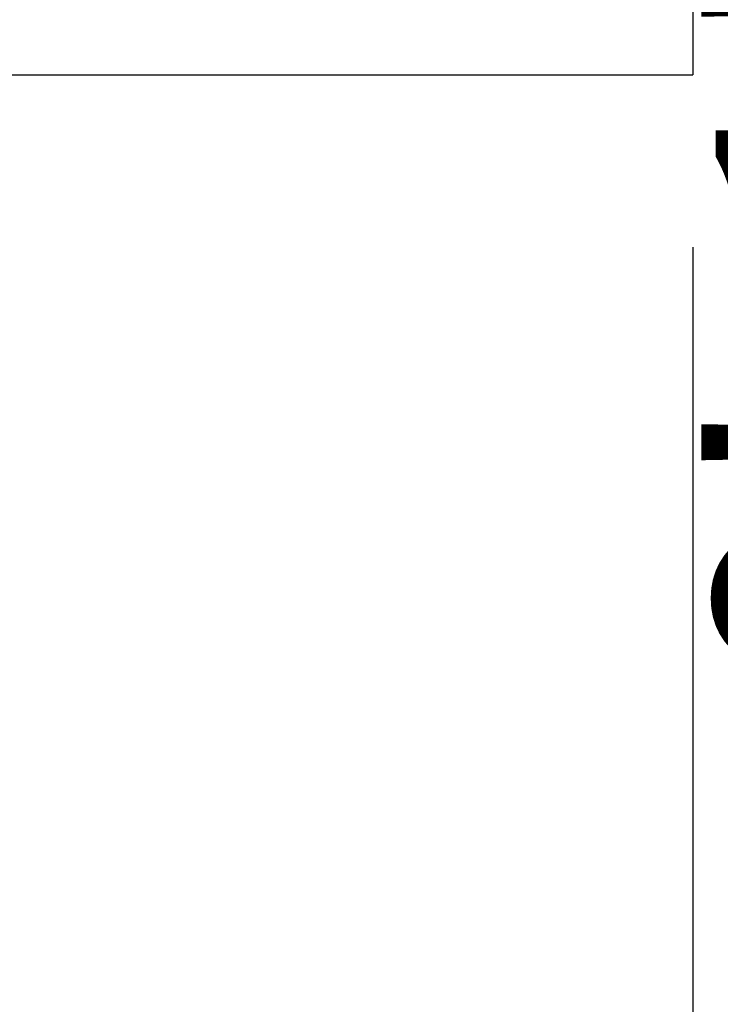
# Model space of a CAD drawing. Units: millimetres. Extents: x 7894 to 8038, y 6851 to 6951.
# Tile 12 of 49: x 7978.394 to 7980.935, y 6875.21 to 6878.784. Entities that reach past the tile are written whole.
import ezdxf

# ---------------------------------------------------------------- set-up
doc = ezdxf.new("R2010")
doc.units = ezdxf.units.MM
doc.layers.add('A-ANNO-DIMS', color=2, linetype='Continuous', lineweight=18)
doc.layers.add('A-FURN-SHLF', color=7, linetype='Continuous', lineweight=30)
doc.styles.get("Standard").update_dxf_attribs({"font": 'arial.ttf'})
doc.dimstyles.new('ISO-25', dxfattribs={"dimtxt": 1, "dimasz": 1, "dimexe": 1.25, "dimexo": 0.625, "dimtad": 1, "dimdec": 0, "dimlunit": 4, "dimtxsty": 'Standard', "dimcen": 2.5, "dimclrt": 1, "dimadec": 0, "dimazin": 0, "dimtfac": 1, "dimtdec": 0, "dimtmove": 0, "dimatfit": 3, "dimfxl": 1, "dimarcsym": 0})

# ---------------------------------------------------------------- blocks, each defined once
blk = doc.blocks.new('*D22')
at = {"layer": 'A-ANNO-DIMS', "color": 0, "lineweight": -2, "transparency": 16777216}
for p, q in [((7983.3131, 6866.2225), (7983.3131, 6876.8981)), ((7981.3426, 6865.2225), (7984.5631, 6865.2225)), ((7983.3131, 6864.7225), (7983.3131, 6865.2225)), ((7981.3426, 6864.7225), (7984.5631, 6864.7225)), ((7983.3131, 6863.7225), (7983.3131, 6862.7225))]:
    blk.add_line(p, q, dxfattribs=at)
at = {"layer": 'A-ANNO-DIMS', "color": 0, "transparency": 16777216}
for points in [[(7983.1464, 6866.2225), (7983.4798, 6866.2225), (7983.3131, 6865.2225)], [(7983.1464, 6863.7225), (7983.4798, 6863.7225), (7983.3131, 6864.7225)]]:
    blk.add_solid(points, dxfattribs=at)
at = {"layer": 'Defpoints', "color": 0, "transparency": 16777216}
for p in [(7980.7176, 6865.2225), (7983.3131, 6865.2225), (7980.7176, 6864.7225)]:
    blk.add_point(p, dxfattribs=at)
at = {"layer": 'A-ANNO-DIMS', "color": 1, "transparency": 16777216, "insert": (7982.171, 6872.0603), "char_height": 1, "attachment_point": 5, "rotation": 90}
blk.add_mtext('0\'-0 1/2" TYP.', dxfattribs=at)
blk = doc.blocks.new('*D36')
at = {"layer": 'A-ANNO-DIMS', "color": 0, "lineweight": -2, "transparency": 16777216}
for p, q in [((7980.8359, 6877.9586), (7980.8359, 6858.5122)), ((7944.4866, 6864.4359), (7944.4866, 6858.5122)), ((7945.4866, 6859.7622), (7979.8359, 6859.7622))]:
    blk.add_line(p, q, dxfattribs=at)
at = {"layer": 'A-ANNO-DIMS', "color": 0, "transparency": 16777216}
for points in [[(7945.4866, 6859.9288), (7945.4866, 6859.5955), (7944.4866, 6859.7622)], [(7979.8359, 6859.9288), (7979.8359, 6859.5955), (7980.8359, 6859.7622)]]:
    blk.add_solid(points, dxfattribs=at)
at = {"layer": 'Defpoints', "color": 0, "transparency": 16777216}
for p in [(7980.8359, 6878.5836), (7944.4866, 6865.0609), (7980.8359, 6859.7622)]:
    blk.add_point(p, dxfattribs=at)
at = {"layer": 'A-ANNO-DIMS', "color": 1, "transparency": 16777216, "insert": (7962.6613, 6860.9046), "char_height": 1, "attachment_point": 5}
blk.add_mtext('3\'-0 1/2"', dxfattribs=at)
blk = doc.blocks.new('*D39')
at = {"layer": 'A-ANNO-DIMS', "color": 0, "lineweight": -2, "transparency": 16777216}
for p, q in [((7982.6834, 6874.8578), (7982.6834, 6879.7661)), ((7964.1574, 6873.8578), (7983.9334, 6873.8578)), ((7982.6834, 6872.9028), (7982.6834, 6873.8578)), ((7981.4609, 6872.9028), (7983.9334, 6872.9028)), ((7982.6834, 6871.9028), (7982.6834, 6870.9028))]:
    blk.add_line(p, q, dxfattribs=at)
at = {"layer": 'A-ANNO-DIMS', "color": 0, "transparency": 16777216}
for points in [[(7982.5168, 6874.8578), (7982.8501, 6874.8578), (7982.6834, 6873.8578)], [(7982.5168, 6871.9028), (7982.8501, 6871.9028), (7982.6834, 6872.9028)]]:
    blk.add_solid(points, dxfattribs=at)
at = {"layer": 'Defpoints', "color": 0, "transparency": 16777216}
for p in [(7963.5324, 6873.8578), (7982.6834, 6873.8578), (7980.8359, 6872.9028)]:
    blk.add_point(p, dxfattribs=at)
at = {"layer": 'A-ANNO-DIMS', "color": 1, "transparency": 16777216, "insert": (7981.5479, 6877.8119), "char_height": 1, "attachment_point": 5, "rotation": 90}
blk.add_mtext('0\'-1"', dxfattribs=at)
blk = doc.blocks.new('*D40')
at = {"layer": 'A-ANNO-DIMS', "color": 0, "lineweight": -2, "transparency": 16777216}
for p, q in [((7982.6834, 6878.5836), (7982.6834, 6885.822)), ((7981.4609, 6878.5836), (7983.9334, 6878.5836)), ((7982.6834, 6874.8578), (7982.6834, 6877.5836)), ((7964.1574, 6873.8578), (7983.9334, 6873.8578))]:
    blk.add_line(p, q, dxfattribs=at)
at = {"layer": 'A-ANNO-DIMS', "color": 0, "transparency": 16777216}
for points in [[(7982.5168, 6877.5836), (7982.8501, 6877.5836), (7982.6834, 6878.5836)], [(7982.5168, 6874.8578), (7982.8501, 6874.8578), (7982.6834, 6873.8578)]]:
    blk.add_solid(points, dxfattribs=at)
at = {"layer": 'Defpoints', "color": 0, "transparency": 16777216}
for p in [(7980.8359, 6878.5836), (7982.6834, 6878.5836), (7963.5324, 6873.8578)]:
    blk.add_point(p, dxfattribs=at)
at = {"layer": 'A-ANNO-DIMS', "color": 1, "transparency": 16777216, "insert": (7981.5414, 6882.7028), "char_height": 1, "attachment_point": 5, "rotation": 90}
blk.add_mtext('0\'-4 1/2"', dxfattribs=at)

msp = doc.modelspace()

# ---------------------------------------------------------------- linework, layer by layer
at = {"layer": 'A-FURN-SHLF'}
for p in [(7980.8359, 6879.0836, -3.5), (7963.5324, 6878.5836, -3.5)]:
    msp.add_line(p, (7980.8359, 6878.5836, -3.5), dxfattribs=at)

# ---------------------------------------------------------------- dimensions: what is measured, and where the dimension line sits
at = {"layer": 'A-ANNO-DIMS'}
for base, p1, p2, picture, middle in [((7982.6834, 6878.5836), (7963.5324, 6873.8578), (7980.8359, 6878.5836), '*D40', (7981.5414, 6882.7028)), ((7982.6834, 6873.8578), (7980.8359, 6872.9028), (7963.5324, 6873.8578), '*D39', (7981.5479, 6877.8119))]:
    dim = msp.add_linear_dim(base=base, p1=p1, p2=p2, angle=90, dimstyle='ISO-25', override={"dimdec": 1, "dimlfac": 1, "dimrnd": 0, "dimzin": 1, "dimdsep": 46, "dimlunit": 4, "dimfrac": 2}, dxfattribs=at)
    dim.commit()
    dim.dimension.update_dxf_attribs({"geometry": picture, "text_midpoint": middle})
dim = msp.add_linear_dim(base=(7980.8359, 6859.7622), p1=(7944.4866, 6865.0609), p2=(7980.8359, 6878.5836), dimstyle='ISO-25', override={"dimdec": 1, "dimlfac": 1, "dimrnd": 0, "dimzin": 1, "dimdsep": 46, "dimlunit": 4, "dimfrac": 2}, dxfattribs=at)
dim.commit()
dim.dimension.update_dxf_attribs({"geometry": '*D36', "text_midpoint": (7962.6613, 6860.9046)})
dim = msp.add_linear_dim(base=(7983.3131, 6865.2225), p1=(7980.7176, 6864.7225), p2=(7980.7176, 6865.2225), angle=90, text='<> TYP.', dimstyle='ISO-25', override={"dimdec": 1, "dimlfac": 1, "dimrnd": 0, "dimzin": 1, "dimdsep": 46, "dimlunit": 4, "dimfrac": 2}, dxfattribs=at)
dim.commit()
dim.dimension.update_dxf_attribs({"geometry": '*D22', "text_midpoint": (7982.171, 6872.0603)})

doc.saveas('drawing.dxf')
